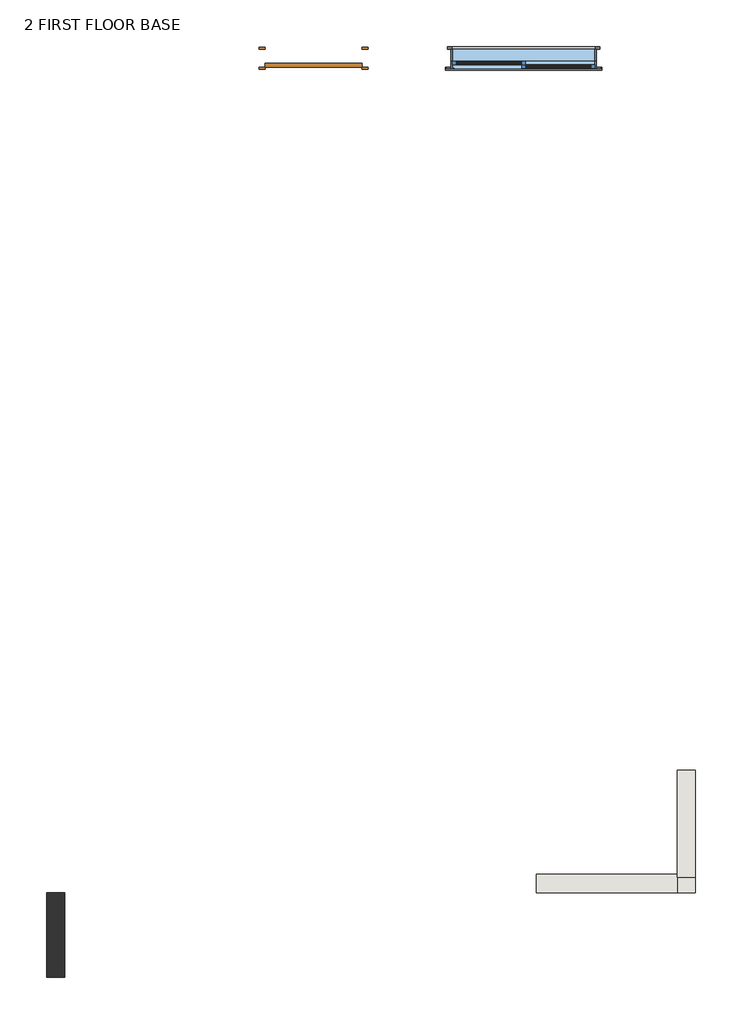
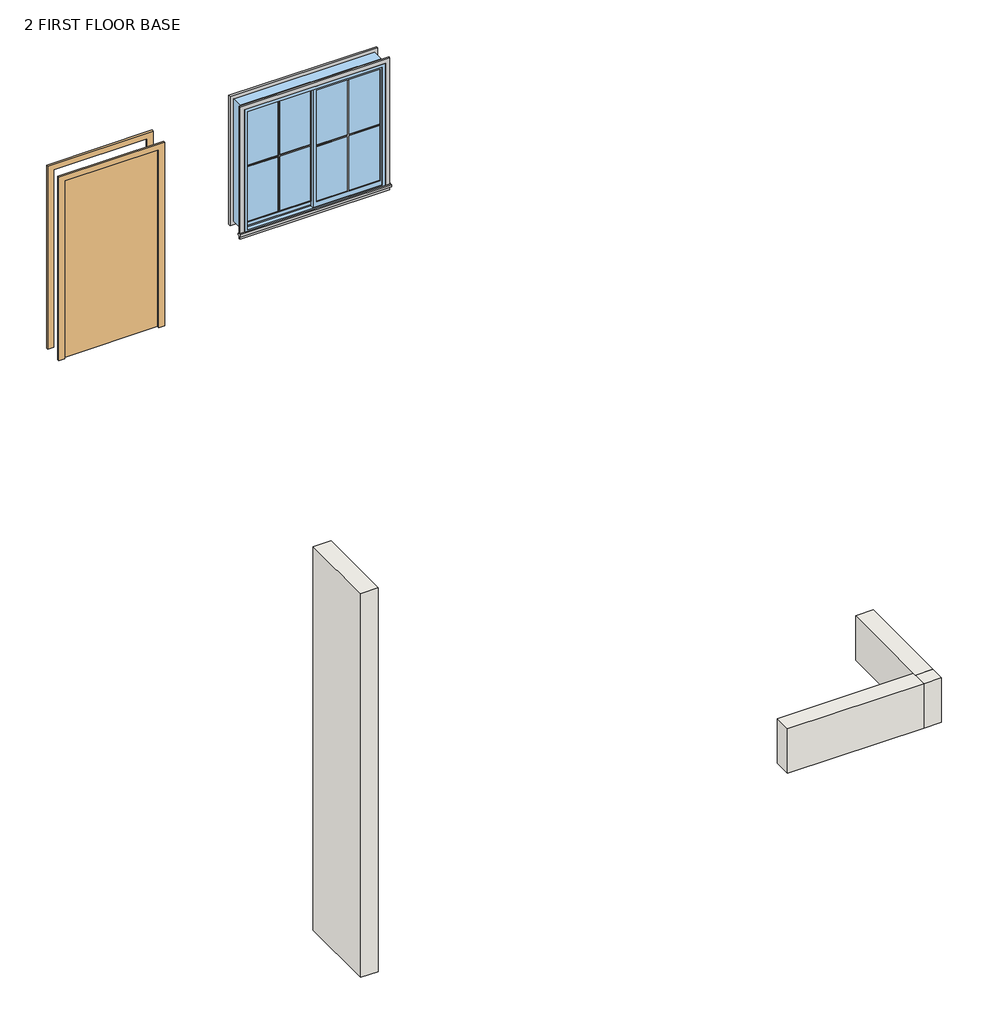
# One storey: 4 proxies, 4 walls, 1 door, 1 window.
"""IFC4 building model written with IfcOpenShell, lengths in millimetres."""

from ifc_helpers import new_model, si_unit, frame, origin, place, context, project, spatial, polyline, outline, extrude, faceted_brep, transform, mapped, element, save
from components import muntin_pattern_2x2_muntin_pattern_2x2_52b72501, trim_window_exterior_flat_with_sill_c98b2dec, trim_window_interior_flat_picture_frame_b05ee221, single_flush_md_e3fbe821, window_sliding_double_89c6b595

model = new_model("IFC4")

# Units and contexts
model_context = context("Model", 3, world=origin())
ifc_project = project(units=[si_unit("LENGTHUNIT", "METRE", prefix="MILLI")], contexts=[model_context])

# Site, building, storey
site = spatial("IfcSite", under=ifc_project)
building = spatial("IfcBuilding", under=site)
storey = spatial("IfcBuildingStorey", under=building, Name="2 FIRST FLOOR BASE", Elevation=3352.8)

# Proxies
placement = place(None, origin())
muntin_pattern_2x2_muntin_pattern_2x2_shape = muntin_pattern_2x2_muntin_pattern_2x2_52b72501(model_context)
element("IfcBuildingElementProxy", 1, Name="Muntin Pattern_2x2 : Muntin Pattern_2x2", ObjectType="Muntin Pattern_2x2 : Muntin Pattern_2x2", at=placement, inside=storey, context=model_context, shape_type="MappedRepresentation", body=[
    mapped(muntin_pattern_2x2_muntin_pattern_2x2_shape, transform((475.7432451, 2460.3284118, 4349.75), x_axis=(-1.0, 0.0, 0.0), y_axis=(0.0, -1.0, 0.0), z_axis=(0.0, 0.0, 1.0))),
])
element("IfcBuildingElementProxy", 2, Name="Muntin Pattern_2x2 : Muntin Pattern_2x2", ObjectType="Muntin Pattern_2x2 : Muntin Pattern_2x2", at=placement, inside=storey, context=model_context, shape_type="MappedRepresentation", body=[
    mapped(muntin_pattern_2x2_muntin_pattern_2x2_shape, transform((1348.8682451, 2415.8784118, 4349.75), x_axis=(-1.0, 0.0, 0.0), y_axis=(0.0, -1.0, 0.0), z_axis=(0.0, 0.0, 1.0))),
])
trim_window_exterior_flat_with_sill_shape = trim_window_exterior_flat_with_sill_c98b2dec(model_context)
element("IfcBuildingElementProxy", 3, Name="Trim-Window-Exterior-Flat : with Sill", ObjectType="Trim-Window-Exterior-Flat : with Sill", at=placement, inside=storey, context=model_context, shape_type="MappedRepresentation", body=[
    mapped(trim_window_exterior_flat_with_sill_shape, transform((912.3057451, 2406.3534118, 5943.6), x_axis=(1.0, 0.0, 0.0), y_axis=(0.0, 0.0, 1.0), z_axis=(0.0, -1.0, 0.0))),
])
trim_window_interior_flat_picture_frame_shape = trim_window_interior_flat_picture_frame_b05ee221(model_context)
element("IfcBuildingElementProxy", 4, Name="Trim-Window-Interior-Flat : Picture Frame", ObjectType="Trim-Window-Interior-Flat : Picture Frame", at=placement, inside=storey, context=model_context, shape_type="MappedRepresentation", body=[
    mapped(trim_window_interior_flat_picture_frame_shape, transform((912.3057451, 2634.9534118, 5943.6), x_axis=(-1.0, 0.0, 0.0), y_axis=(0.0, 0.0, 1.0), z_axis=(0.0, 1.0, 0.0))),
])

# Door
single_flush_md_shape = single_flush_md_e3fbe821(model_context)
element("IfcDoor", 5, ObjectType="Single-Flush : MD", at=placement, inside=storey, context=model_context, shape_type="MappedRepresentation", body=[
    mapped(single_flush_md_shape, transform((-1729.2942549, 2520.6534118, 3352.8), x_axis=(-1.0, 0.0, 0.0), y_axis=(0.0, -1.0, 0.0), z_axis=(0.0, 0.0, 1.0))),
])

# Walls
element("IfcWall", 6, ObjectType="9\"", at=placement, inside=storey, context=model_context, shape_type="SweptSolid", body=[
    extrude(outline(polyline([(2842.7057451, -7770.558484), (2842.7057451, -6427.4296941), (3071.3057451, -6427.4296941), (3071.3057451, -7770.558484), (2842.7057451, -7770.558484)])), frame((0.0, 0.0, 2743.2), z_axis=(0.0, 0.0, 1.0), x_axis=(1.0, 0.0, 0.0)), (0.0, 0.0, 1.0), 609.6),
])
element("IfcWall", 7, ObjectType="9\"", at=placement, inside=storey, context=model_context, shape_type="Brep", body=[
    faceted_brep([(2842.7057451, -7732.458484, 2743.2), (1072.9478614, -7732.458484, 2743.2), (1072.9478614, -7732.458484, 3352.8), (2842.7057451, -7732.458484, 3352.8), (2842.7057451, -7961.058484, 2743.2), (2842.7057451, -7961.058484, 3352.8), (1072.9478614, -7961.058484, 3352.8), (1072.9478614, -7961.058484, 2743.2), (2842.7057451, -7770.558484, 2743.2), (2842.7057451, -7770.558484, 3352.8)], [[[0, 1, 2, 3]], [[4, 5, 6, 7]], [[1, 0, 8, 4, 7]], [[2, 1, 7, 6]], [[3, 2, 6, 5, 9]], [[0, 3, 9, 5, 4, 8]]]),
])
element("IfcWall", 8, ObjectType="9\"", at=placement, inside=storey, context=model_context, shape_type="Brep", body=[
    faceted_brep([(-5084.2350579, -7961.058484, 8007.3851299), (-5084.2350579, -7961.058484, 6705.6), (-5084.2350579, -7961.058484, 3505.2), (-5084.2350579, -7961.058484, 3352.8), (-5084.2350579, -7961.058484, 2743.2), (-5084.2350579, -9027.858484, 2743.2), (-5084.2350579, -9027.858484, 8007.3851299), (-4855.6350579, -7961.058484, 2743.2), (-4855.6350579, -7961.058484, 8007.3851299), (-4855.6350579, -9027.858484, 8007.3851299), (-4855.6350579, -9027.858484, 2743.2)], [[[0, 1, 2, 3, 4, 5, 6]], [[7, 8, 9, 10]], [[5, 4, 7, 10]], [[6, 5, 10, 9]], [[0, 6, 9, 8]], [[0, 8, 7, 4, 3, 2, 1]]]),
])
element("IfcWall", 9, ObjectType="9\"", at=placement, inside=storey, context=model_context, shape_type="SweptSolid", body=[
    extrude(outline(polyline([(2842.7057451, -7961.058484), (2842.7057451, -7770.558484), (3071.3057451, -7770.558484), (3071.3057451, -7961.058484), (2842.7057451, -7961.058484)])), frame((0.0, 0.0, 2743.2), z_axis=(0.0, 0.0, 1.0), x_axis=(1.0, 0.0, 0.0)), (0.0, 0.0, 1.0), 609.6),
])

# Window
window_sliding_double_shape = window_sliding_double_89c6b595(model_context)
element("IfcWindow", 10, ObjectType="Window-Sliding-Double", at=placement, inside=storey, context=model_context, shape_type="MappedRepresentation", body=[
    mapped(window_sliding_double_shape, transform((912.3057451, 2516.8434118, 3352.8), x_axis=(-1.0, 0.0, 0.0), y_axis=(0.0, -1.0, 0.0), z_axis=(0.0, 0.0, 1.0))),
])

save(model, "model.ifc")

# Revit data of these elements
# Type "Muntin Pattern_2x2 : Muntin Pattern_2x2"
#   Width [instance default] = 4' - 0"
#   Thickness = 0' - 0 1/2"
#   Height [instance default] = 4' - 0"
#   Distance = 0' - 0 3/4"
#   Interior Material [instance default] = none
#   Exterior Material [instance default] = none
#   Default Elevation = 0
# Type "Trim-Window-Exterior-Flat : with Sill"
#   Trim Width = 0' - 2 1/4"
#   Trim Thickness_Picture Frame = 0' - 1 1/4"
#   Trim Thickness_with Sill = 0' - 0 3/4"
#   Sill Thickness = 0' - 1 1/4"
#   Opening Width [instance default] = 2' - 0"
#   Opening Height [instance default] = 3' - 0"
#   Default Elevation = 4' - 0"
#   Sill = yes
#   Picture Frame = no
#   Trim Material [instance default] = none
# Type "Trim-Window-Interior-Flat : Picture Frame"
#   Trim Thickness_Picture Frame = 0' - 1 1/4"
#   Trim Width = 0' - 2 1/4"
#   Trim Thickness_with Sill = 0' - 0 3/4"
#   Sill Thickness = 0' - 1 1/4"
#   Opening Width [instance default] = 2' - 0"
#   Opening Height [instance default] = 3' - 0"
#   Default Elevation = 4' - 0"
#   Sill = no
#   Picture Frame = yes
#   Trim Material [instance default] = none
# Type "Single-Flush : MD"
#   Type Mark = "10"
#   Construction Type Id = "MDOOR"
#   Assembly Code = "C1020"
#   Analytic Construction = "Metal"
#   Thickness = 0' - 2"
#   Heat Transfer Coefficient (U) = 0.651978 BTU/(h·ft²·°F)
#   Height = 8' - 0"
#   Trim Projection Ext = 0' - 1"
#   Trim Projection Int = 0' - 1"
#   Trim Width = 0' - 3"
#   Width = 4' - 0"
#   Define Thermal Properties by = 1
#   Door Material = Door - Panel
#   Frame Material = Door - Frame
#   Visual Light Transmittance = 0
#   Solar Heat Gain Coefficient = 0
#   Function = (empty or 0)
#   Wall Closure = (empty or 0)
# Type "9\""
#   Assembly Code = "B2010"
#   Layers, outside or top first: 0' - 9" no material (function 1)
# Type "Window-Sliding-Double"
#   Type Mark = "19"
#   Fire Rating = "0.5h"
#   Assembly Code = "B2020100"
#   Analytic Construction = "Double glazing - domestic"
#   Window Inset [instance default] = 0' - 0"
#   Wall Thickness [instance default] = 0' - 6"
#   Visual Light Transmittance = 0.81
#   Thermal Resistance (R) = 1.8146 (h·ft²·°F)/BTU
#   Solar Heat Gain Coefficient = 0.76
#   Muntin Width = 2' - 8 5/8"
#   Muntin Height = 5' - 0 1/4"
#   Interior Wall Closure [instance default] = 0' - 2 3/4"
#   Heat Transfer Coefficient (U) = 0.5511 BTU/(h·ft²·°F)
#   Frame Extension [instance default] = 0' - 0 1/4"
#   Exterior Wall Closure [instance default] = 0' - 1 1/4"
#   Rough Width = 6' - 0 1/2"
#   Rough Height = 5' - 6 1/2"
#   Height = 5' - 6"
#   Extension Jamb [instance default] = 0' - 2 3/4"
#   Default Sill Height = 3' - 0"
#   Width = 6' - 0"
#   Interior Trim Visibility [instance default] = yes
#   Indicator Visibility [instance default] = yes
#   Exterior Trim Visibility [instance default] = yes
#   Muntin Visibility = yes
#   Extension Jamb Visibility [instance default] = yes
#   Muntin Pattern = Muntin Pattern_2x2 : Muntin Pattern_2x2
#   Interior Trim Material = Wood - Stained
#   Interior Trim = Trim-Window-Interior-Flat : Picture Frame
#   Interior Frame Material = Wood - Stained
#   Glass Panel Material = Glass
#   Exterior Trim Material = Clad - White
#   Exterior Trim = Trim-Window-Exterior-Flat : with Sill
#   Exterior Frame Material = Clad - White
#   Wall Closure = (empty or 0)
# Elements 1, 2 (IfcBuildingElementProxy, "Muntin Pattern_2x2 : Muntin Pattern_2x2")
#   Width = 2' - 8 5/8"
#   Height = 5' - 0 1/4"
#   Interior Material = Wood - Stained
#   Exterior Material = Clad - White
#   Phase Created = New Construction
#   Materials on its faces: "Clad - White", "Wood - Stained"
# Element 3 (IfcBuildingElementProxy, "Trim-Window-Exterior-Flat : with Sill")
#   Opening Width = 6' - 0"
#   Opening Height = 5' - 6"
#   Trim Material = Clad - White
#   Phase Created = New Construction
#   Materials on its faces: "Clad - White"
# Element 4 (IfcBuildingElementProxy, "Trim-Window-Interior-Flat : Picture Frame")
#   Opening Width = 6' - 0"
#   Opening Height = 5' - 6"
#   Trim Material = Wood - Stained
#   Phase Created = New Construction
#   Materials on its faces: "Wood - Stained"
# Element 5 (IfcDoor, "Single-Flush : MD")
#   Phase Created = New Construction
#   Materials on its faces: "Door - Frame", "Door - Panel"
# Elements 6, 7, 9 (IfcWall, "9\"")
#   built-in parameter 1001111 = -2' - 0"
#   Top Offset = 0' - 0"
#   Base Offset = -2' - 0"
#   Unconnected Height = 2' - 0"
#   wall height = 2' - 0"
#   Phase Created = New Construction
#   Base Constraint = 2 FIRST FLOOR BASE
#   Materials on its faces: "Default Wall", "outer wall"
# Element 8 (IfcWall, "9\"")
#   built-in parameter 1001111 = -2' - 0"
#   Top Offset = 4' - 3.25138"
#   Base Offset = -2' - 0"
#   wall height = 17' - 3.25138"
#   Phase Created = New Construction
#   Base Constraint = 2 FIRST FLOOR BASE
#   Top Constraint = 4 SECOND FLOOR BASE
#   Materials on its faces: "st wall(1)", "Default Wall"
# Element 10 (IfcWindow, "Window-Sliding-Double")
#   Mark = "8"
#   Window Inset = 0' - 0"
#   Interior Wall Closure = 0' - 2 3/4"
#   Frame Extension = 0' - 0 1/4"
#   Exterior Wall Closure = 0' - 1 1/4"
#   Interior Trim Visibility = yes
#   Indicator Visibility = yes
#   Exterior Trim Visibility = yes
#   Phase Created = New Construction
#   Materials on its faces: "Wood - Stained", "Glass", "Clad - White"
# Materials
#   "Door - Panel": class "Wood", colour RGB 210 159 95, transparency 0, Cost = 0
#   "Door - Frame": colour RGB 118 70 51, transparency 0, Cost = 0
#   "Wood - Stained": class "Wood", colour RGB 224 178 126, transparency 0, Cost = 0
#   "Glass": class "Glass", colour RGB 0 128 192, transparency 0.75, Description = "Soda Lime Glass", Cost = 0
#   "Clad - White": class "Wood", colour RGB 242 242 238, transparency 0, Cost = 0
#   "Default Wall": colour RGB 128 128 128, transparency 0, Cost = 0
#   "outer wall": class "Generic", colour RGB 85 88 91, transparency 0, Cost = 0
#   "st wall(1)": class "Generic", colour RGB 173 147 123, transparency 0, Cost = 0
